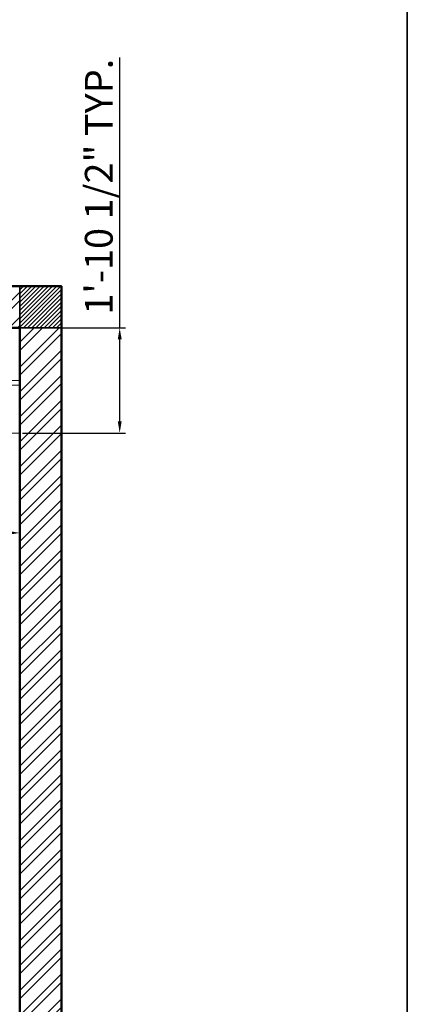
# Model space of a CAD drawing. Units: millimetres. Extents: x 20768 to 23556, y 50760 to 52704.
# Tile 29 of 36: x 21551 to 21634, y 52368 to 52580. Entities that reach past the tile are written whole.
import ezdxf

# ---------------------------------------------------------------- set-up
doc = ezdxf.new("R2010")
doc.units = ezdxf.units.MM
for name, color, linetype, lineweight in [('A-ANNO-TTLB', 7, 'Continuous', 35), ('A-FURN', 8, 'Continuous', 18), ('A-WALL', 7, 'Continuous', 50), ('A-WALL-PATT', 8, 'Continuous', 13), ('S-ANNO-DIMS', 2, 'Continuous', 18), ('S-COLS', 20, 'Continuous', 35)]:
    doc.layers.add(name, color=color, linetype=linetype, lineweight=lineweight)
doc.styles.get("Standard").update_dxf_attribs({"font": 'arial.ttf'})
doc.dimstyles.new('ISO-25', dxfattribs={"dimtxt": 6, "dimasz": 2.5, "dimexe": 1.25, "dimexo": 0.625, "dimtad": 1, "dimdec": 0, "dimlunit": 3, "dimtxsty": 'Standard', "dimcen": 2.5, "dimadec": 0, "dimazin": 0, "dimtfac": 1, "dimtdec": 0, "dimtmove": 0, "dimatfit": 3, "dimfxl": 1, "dimarcsym": 0})
pattern_1 = [(45, (-37.4434, 0), (-2.69407684, 2.69407684), []), (45, (-35.6473, 0), (-2.69407684, 2.69407684), [])]

# ---------------------------------------------------------------- blocks, each defined once
blk = doc.blocks.new('wb')
for p, q in [((21205.25, 52502.52), (21061.44, 52502.52)), ((21205.25, 52501.52), (21061.44, 52501.52))]:
    blk.add_line(p, q)
blk.add_lwpolyline([(21205.25, 52513.9), (21061.44, 52513.9), (21061.44, 52491.15), (21205.25, 52491.15)], close=True)
for points in [[(21064.45, 52510.07, 0.695903), (21063.5, 52509.77), (21063.75, 52508.98), (21064.7, 52509.27)], [(21067.97, 52510.07, 0.695903), (21067.01, 52509.77), (21067.26, 52508.98), (21068.21, 52509.27)], [(21071.48, 52510.07, 0.695903), (21070.52, 52509.77), (21070.77, 52508.98), (21071.73, 52509.27)], [(21074.99, 52510.07, 0.695903), (21074.04, 52509.77), (21074.28, 52508.98), (21075.24, 52509.27)], [(21078.5, 52510.07, 0.695903), (21077.55, 52509.77), (21077.8, 52508.98), (21078.75, 52509.27)], [(21082.02, 52510.07, 0.695903), (21081.06, 52509.77), (21081.31, 52508.98), (21082.26, 52509.27)], [(21085.53, 52510.07, 0.695903), (21084.57, 52509.77), (21084.82, 52508.98), (21085.78, 52509.27)], [(21089.04, 52510.07, 0.695903), (21088.09, 52509.77), (21088.33, 52508.98), (21089.29, 52509.27)], [(21092.55, 52510.07, 0.695903), (21091.6, 52509.77), (21091.85, 52508.98), (21092.8, 52509.27)], [(21096.07, 52510.07, 0.695903), (21095.11, 52509.77), (21095.36, 52508.98), (21096.31, 52509.27)], [(21099.58, 52510.07, 0.695903), (21098.62, 52509.77), (21098.87, 52508.98), (21099.83, 52509.27)], [(21103.09, 52510.07, 0.695903), (21102.14, 52509.77), (21102.38, 52508.98), (21103.34, 52509.27)], [(21106.6, 52510.07, 0.695903), (21105.65, 52509.77), (21105.9, 52508.98), (21106.85, 52509.27)], [(21110.12, 52510.07, 0.695903), (21109.16, 52509.77), (21109.41, 52508.98), (21110.36, 52509.27)], [(21113.63, 52510.07, 0.695903), (21112.67, 52509.77), (21112.92, 52508.98), (21113.88, 52509.27)], [(21117.14, 52510.07, 0.695903), (21116.19, 52509.77), (21116.43, 52508.98), (21117.39, 52509.27)], [(21120.65, 52510.07, 0.695903), (21119.7, 52509.77), (21119.95, 52508.98), (21120.9, 52509.27)], [(21124.17, 52510.07, 0.695903), (21123.21, 52509.77), (21123.46, 52508.98), (21124.41, 52509.27)], [(21127.68, 52510.07, 0.695903), (21126.72, 52509.77), (21126.97, 52508.98), (21127.93, 52509.27)], [(21131.19, 52510.07, 0.695903), (21130.24, 52509.77), (21130.48, 52508.98), (21131.44, 52509.27)], [(21134.7, 52510.07, 0.695903), (21133.75, 52509.77), (21134, 52508.98), (21134.95, 52509.27)], [(21138.22, 52510.07, 0.695903), (21137.26, 52509.77), (21137.51, 52508.98), (21138.46, 52509.27)], [(21141.73, 52510.07, 0.695903), (21140.77, 52509.77), (21141.02, 52508.98), (21141.98, 52509.27)], [(21145.24, 52510.07, 0.695903), (21144.29, 52509.77), (21144.54, 52508.98), (21145.49, 52509.27)], [(21148.75, 52510.07, 0.695903), (21147.8, 52509.77), (21148.05, 52508.98), (21149, 52509.27)], [(21152.27, 52510.07, 0.695903), (21151.31, 52509.77), (21151.56, 52508.98), (21152.52, 52509.27)], [(21155.78, 52510.07, 0.695903), (21154.83, 52509.77), (21155.07, 52508.98), (21156.03, 52509.27)], [(21159.29, 52510.07, 0.695903), (21158.34, 52509.77), (21158.59, 52508.98), (21159.54, 52509.27)], [(21162.8, 52510.07, 0.695903), (21161.85, 52509.77), (21162.1, 52508.98), (21163.05, 52509.27)], [(21166.32, 52510.07, 0.695903), (21165.36, 52509.77), (21165.61, 52508.98), (21166.57, 52509.27)], [(21169.83, 52510.07, 0.695903), (21168.88, 52509.77), (21169.12, 52508.98), (21170.08, 52509.27)], [(21173.34, 52510.07, 0.695903), (21172.39, 52509.77), (21172.64, 52508.98), (21173.59, 52509.27)], [(21176.86, 52510.07, 0.695903), (21175.9, 52509.77), (21176.15, 52508.98), (21177.1, 52509.27)], [(21180.37, 52510.07, 0.695903), (21179.41, 52509.77), (21179.66, 52508.98), (21180.62, 52509.27)], [(21183.88, 52510.07, 0.695903), (21182.93, 52509.77), (21183.17, 52508.98), (21184.13, 52509.27)], [(21187.39, 52510.07, 0.695903), (21186.44, 52509.77), (21186.69, 52508.98), (21187.64, 52509.27)], [(21190.91, 52510.07, 0.695903), (21189.95, 52509.77), (21190.2, 52508.98), (21191.15, 52509.27)], [(21194.42, 52510.07, 0.695903), (21193.46, 52509.77), (21193.71, 52508.98), (21194.67, 52509.27)], [(21197.93, 52510.07, 0.695903), (21196.98, 52509.77), (21197.22, 52508.98), (21198.18, 52509.27)], [(21068.81, 52496.1), (21067.85, 52495.8), (21068.19, 52494.73, 1), (21069.14, 52495.03)], [(21072.32, 52496.1), (21071.37, 52495.8), (21071.7, 52494.73, 1), (21072.65, 52495.03)], [(21075.83, 52496.1), (21074.88, 52495.8), (21075.21, 52494.73, 1), (21076.17, 52495.03)], [(21079.35, 52496.1), (21078.39, 52495.8), (21078.73, 52494.73, 1), (21079.68, 52495.03)], [(21082.86, 52496.1), (21081.9, 52495.8), (21082.24, 52494.73, 1), (21083.19, 52495.03)], [(21086.37, 52496.1), (21085.42, 52495.8), (21085.75, 52494.73, 1), (21086.7, 52495.03)], [(21089.88, 52496.1), (21088.93, 52495.8), (21089.26, 52494.73, 1), (21090.22, 52495.03)], [(21093.4, 52496.1), (21092.44, 52495.8), (21092.78, 52494.73, 1), (21093.73, 52495.03)], [(21096.91, 52496.1), (21095.95, 52495.8), (21096.29, 52494.73, 1), (21097.24, 52495.03)], [(21100.42, 52496.1), (21099.47, 52495.8), (21099.8, 52494.73, 1), (21100.76, 52495.03)], [(21103.93, 52496.1), (21102.98, 52495.8), (21103.31, 52494.73, 1), (21104.27, 52495.03)], [(21107.45, 52496.1), (21106.49, 52495.8), (21106.83, 52494.73, 1), (21107.78, 52495.03)], [(21110.96, 52496.1), (21110, 52495.8), (21110.34, 52494.73, 1), (21111.29, 52495.03)], [(21114.47, 52496.1), (21113.52, 52495.8), (21113.85, 52494.73, 1), (21114.81, 52495.03)], [(21117.98, 52496.1), (21117.03, 52495.8), (21117.36, 52494.73, 1), (21118.32, 52495.03)], [(21121.5, 52496.1), (21120.54, 52495.8), (21120.88, 52494.73, 1), (21121.83, 52495.03)], [(21125.01, 52496.1), (21124.05, 52495.8), (21124.39, 52494.73, 1), (21125.34, 52495.03)], [(21128.52, 52496.1), (21127.57, 52495.8), (21127.9, 52494.73, 1), (21128.86, 52495.03)], [(21132.03, 52496.1), (21131.08, 52495.8), (21131.41, 52494.73, 1), (21132.37, 52495.03)], [(21135.55, 52496.1), (21134.59, 52495.8), (21134.93, 52494.73, 1), (21135.88, 52495.03)], [(21139.06, 52496.1), (21138.1, 52495.8), (21138.44, 52494.73, 1), (21139.39, 52495.03)], [(21142.57, 52496.1), (21141.62, 52495.8), (21141.95, 52494.73, 1), (21142.91, 52495.03)], [(21146.08, 52496.1), (21145.13, 52495.8), (21145.46, 52494.73, 1), (21146.42, 52495.03)], [(21149.6, 52496.1), (21148.64, 52495.8), (21148.98, 52494.73, 1), (21149.93, 52495.03)], [(21153.11, 52496.1), (21152.15, 52495.8), (21152.49, 52494.73, 1), (21153.44, 52495.03)], [(21156.62, 52496.1), (21155.67, 52495.8), (21156, 52494.73, 1), (21156.96, 52495.03)], [(21160.13, 52496.1), (21159.18, 52495.8), (21159.51, 52494.73, 1), (21160.47, 52495.03)], [(21163.65, 52496.1), (21162.69, 52495.8), (21163.03, 52494.73, 1), (21163.98, 52495.03)], [(21167.16, 52496.1), (21166.2, 52495.8), (21166.54, 52494.73, 1), (21167.49, 52495.03)], [(21170.67, 52496.1), (21169.72, 52495.8), (21170.05, 52494.73, 1), (21171.01, 52495.03)], [(21174.18, 52496.1), (21173.23, 52495.8), (21173.56, 52494.73, 1), (21174.52, 52495.03)], [(21177.7, 52496.1), (21176.74, 52495.8), (21177.08, 52494.73, 1), (21178.03, 52495.03)], [(21181.21, 52496.1), (21180.25, 52495.8), (21180.59, 52494.73, 1), (21181.54, 52495.03)], [(21184.72, 52496.1), (21183.77, 52495.8), (21184.1, 52494.73, 1), (21185.06, 52495.03)], [(21188.23, 52496.1), (21187.28, 52495.8), (21187.61, 52494.73, 1), (21188.57, 52495.03)], [(21191.75, 52496.1), (21190.79, 52495.8), (21191.13, 52494.73, 1), (21192.08, 52495.03)], [(21195.26, 52496.1), (21194.31, 52495.8), (21194.64, 52494.73, 1), (21195.59, 52495.03)], [(21198.77, 52496.1), (21197.82, 52495.8), (21198.15, 52494.73, 1), (21199.11, 52495.03)], [(21202.29, 52496.1), (21201.33, 52495.8), (21201.67, 52494.73, 1), (21202.62, 52495.03)]]:
    blk.add_lwpolyline(points, format="xyb", close=True)
for points in [[(21065.76, 52502.52), (21063.98, 52508.23), (21064.93, 52508.53), (21066.81, 52502.52)], [(21069.27, 52502.52), (21067.49, 52508.23), (21068.44, 52508.53), (21070.32, 52502.52)], [(21072.78, 52502.52), (21071, 52508.23), (21071.96, 52508.53), (21073.83, 52502.52)], [(21076.3, 52502.52), (21074.51, 52508.23), (21075.47, 52508.53), (21077.34, 52502.52)], [(21079.81, 52502.52), (21078.03, 52508.23), (21078.98, 52508.53), (21080.86, 52502.52)], [(21083.32, 52502.52), (21081.54, 52508.23), (21082.49, 52508.53), (21084.37, 52502.52)], [(21086.83, 52502.52), (21085.05, 52508.23), (21086.01, 52508.53), (21087.88, 52502.52)], [(21090.35, 52502.52), (21088.57, 52508.23), (21089.52, 52508.53), (21091.39, 52502.52)], [(21093.86, 52502.52), (21092.08, 52508.23), (21093.03, 52508.53), (21094.91, 52502.52)], [(21097.37, 52502.52), (21095.59, 52508.23), (21096.55, 52508.53), (21098.42, 52502.52)], [(21100.88, 52502.52), (21099.1, 52508.23), (21100.06, 52508.53), (21101.93, 52502.52)], [(21104.4, 52502.52), (21102.62, 52508.23), (21103.57, 52508.53), (21105.44, 52502.52)], [(21107.91, 52502.52), (21106.13, 52508.23), (21107.08, 52508.53), (21108.96, 52502.52)], [(21111.42, 52502.52), (21109.64, 52508.23), (21110.6, 52508.53), (21112.47, 52502.52)], [(21114.93, 52502.52), (21113.15, 52508.23), (21114.11, 52508.53), (21115.98, 52502.52)], [(21118.45, 52502.52), (21116.67, 52508.23), (21117.62, 52508.53), (21119.49, 52502.52)], [(21121.96, 52502.52), (21120.18, 52508.23), (21121.13, 52508.53), (21123.01, 52502.52)], [(21125.47, 52502.52), (21123.69, 52508.23), (21124.65, 52508.53), (21126.52, 52502.52)], [(21128.98, 52502.52), (21127.2, 52508.23), (21128.16, 52508.53), (21130.03, 52502.52)], [(21132.5, 52502.52), (21130.72, 52508.23), (21131.67, 52508.53), (21133.54, 52502.52)], [(21136.01, 52502.52), (21134.23, 52508.23), (21135.18, 52508.53), (21137.06, 52502.52)], [(21139.52, 52502.52), (21137.74, 52508.23), (21138.7, 52508.53), (21140.57, 52502.52)], [(21143.03, 52502.52), (21141.25, 52508.23), (21142.21, 52508.53), (21144.08, 52502.52)], [(21146.55, 52502.52), (21144.77, 52508.23), (21145.72, 52508.53), (21147.59, 52502.52)], [(21150.06, 52502.52), (21148.28, 52508.23), (21149.23, 52508.53), (21151.11, 52502.52)], [(21153.57, 52502.52), (21151.79, 52508.23), (21152.75, 52508.53), (21154.62, 52502.52)], [(21157.08, 52502.52), (21155.3, 52508.23), (21156.26, 52508.53), (21158.13, 52502.52)], [(21160.6, 52502.52), (21158.82, 52508.23), (21159.77, 52508.53), (21161.64, 52502.52)], [(21164.11, 52502.52), (21162.33, 52508.23), (21163.28, 52508.53), (21165.16, 52502.52)], [(21167.62, 52502.52), (21165.84, 52508.23), (21166.8, 52508.53), (21168.67, 52502.52)], [(21171.13, 52502.52), (21169.35, 52508.23), (21170.31, 52508.53), (21172.18, 52502.52)], [(21174.65, 52502.52), (21172.87, 52508.23), (21173.82, 52508.53), (21175.69, 52502.52)], [(21178.16, 52502.52), (21176.38, 52508.23), (21177.33, 52508.53), (21179.21, 52502.52)], [(21181.67, 52502.52), (21179.89, 52508.23), (21180.85, 52508.53), (21182.72, 52502.52)], [(21185.19, 52502.52), (21183.4, 52508.23), (21184.36, 52508.53), (21186.23, 52502.52)], [(21188.7, 52502.52), (21186.92, 52508.23), (21187.87, 52508.53), (21189.75, 52502.52)], [(21192.21, 52502.52), (21190.43, 52508.23), (21191.38, 52508.53), (21193.26, 52502.52)], [(21195.72, 52502.52), (21193.94, 52508.23), (21194.9, 52508.53), (21196.77, 52502.52)], [(21199.24, 52502.52), (21197.46, 52508.23), (21198.41, 52508.53), (21200.28, 52502.52)], [(21066.07, 52501.52), (21067.54, 52496.81), (21068.49, 52497.1), (21067.12, 52501.52)], [(21069.58, 52501.52), (21071.05, 52496.81), (21072.01, 52497.1), (21070.63, 52501.52)], [(21073.09, 52501.52), (21074.57, 52496.81), (21075.52, 52497.1), (21074.14, 52501.52)], [(21076.61, 52501.52), (21078.08, 52496.81), (21079.03, 52497.1), (21077.65, 52501.52)], [(21080.12, 52501.52), (21081.59, 52496.81), (21082.55, 52497.1), (21081.17, 52501.52)], [(21083.63, 52501.52), (21085.1, 52496.81), (21086.06, 52497.1), (21084.68, 52501.52)], [(21087.14, 52501.52), (21088.62, 52496.81), (21089.57, 52497.1), (21088.19, 52501.52)], [(21090.66, 52501.52), (21092.13, 52496.81), (21093.08, 52497.1), (21091.7, 52501.52)], [(21094.17, 52501.52), (21095.64, 52496.81), (21096.6, 52497.1), (21095.22, 52501.52)], [(21097.68, 52501.52), (21099.15, 52496.81), (21100.11, 52497.1), (21098.73, 52501.52)], [(21101.2, 52501.52), (21102.67, 52496.81), (21103.62, 52497.1), (21102.24, 52501.52)], [(21104.71, 52501.52), (21106.18, 52496.81), (21107.13, 52497.1), (21105.76, 52501.52)], [(21108.22, 52501.52), (21109.69, 52496.81), (21110.65, 52497.1), (21109.27, 52501.52)], [(21111.73, 52501.52), (21113.2, 52496.81), (21114.16, 52497.1), (21112.78, 52501.52)], [(21115.25, 52501.52), (21116.72, 52496.81), (21117.67, 52497.1), (21116.29, 52501.52)], [(21118.76, 52501.52), (21120.23, 52496.81), (21121.18, 52497.1), (21119.81, 52501.52)], [(21122.27, 52501.52), (21123.74, 52496.81), (21124.7, 52497.1), (21123.32, 52501.52)], [(21125.78, 52501.52), (21127.25, 52496.81), (21128.21, 52497.1), (21126.83, 52501.52)], [(21129.3, 52501.52), (21130.77, 52496.81), (21131.72, 52497.1), (21130.34, 52501.52)], [(21132.81, 52501.52), (21134.28, 52496.81), (21135.23, 52497.1), (21133.86, 52501.52)], [(21136.32, 52501.52), (21137.79, 52496.81), (21138.75, 52497.1), (21137.37, 52501.52)], [(21139.83, 52501.52), (21141.3, 52496.81), (21142.26, 52497.1), (21140.88, 52501.52)], [(21143.35, 52501.52), (21144.82, 52496.81), (21145.77, 52497.1), (21144.39, 52501.52)], [(21146.86, 52501.52), (21148.33, 52496.81), (21149.28, 52497.1), (21147.91, 52501.52)], [(21150.37, 52501.52), (21151.84, 52496.81), (21152.8, 52497.1), (21151.42, 52501.52)], [(21153.88, 52501.52), (21155.35, 52496.81), (21156.31, 52497.1), (21154.93, 52501.52)], [(21157.4, 52501.52), (21158.87, 52496.81), (21159.82, 52497.1), (21158.44, 52501.52)], [(21160.91, 52501.52), (21162.38, 52496.81), (21163.33, 52497.1), (21161.96, 52501.52)], [(21164.42, 52501.52), (21165.89, 52496.81), (21166.85, 52497.1), (21165.47, 52501.52)], [(21167.93, 52501.52), (21169.4, 52496.81), (21170.36, 52497.1), (21168.98, 52501.52)], [(21171.45, 52501.52), (21172.92, 52496.81), (21173.87, 52497.1), (21172.49, 52501.52)], [(21174.96, 52501.52), (21176.43, 52496.81), (21177.38, 52497.1), (21176.01, 52501.52)], [(21178.47, 52501.52), (21179.94, 52496.81), (21180.9, 52497.1), (21179.52, 52501.52)], [(21181.98, 52501.52), (21183.46, 52496.81), (21184.41, 52497.1), (21183.03, 52501.52)], [(21185.5, 52501.52), (21186.97, 52496.81), (21187.92, 52497.1), (21186.54, 52501.52)], [(21189.01, 52501.52), (21190.48, 52496.81), (21191.43, 52497.1), (21190.06, 52501.52)], [(21192.52, 52501.52), (21193.99, 52496.81), (21194.95, 52497.1), (21193.57, 52501.52)], [(21196.03, 52501.52), (21197.51, 52496.81), (21198.46, 52497.1), (21197.08, 52501.52)], [(21199.55, 52501.52), (21201.02, 52496.81), (21201.97, 52497.1), (21200.59, 52501.52)]]:
    blk.add_lwpolyline(points)
blk = doc.blocks.new('*D187')
at = {"layer": 'Defpoints', "color": 0, "transparency": 16777216}
for p in [(21406.93, 52491.15), (21550.74, 52491.15), (21550.74, 52469.58)]:
    blk.add_point(p, dxfattribs=at)
at = {"layer": 'S-ANNO-DIMS', "color": 0, "lineweight": -2, "transparency": 16777216}
for p, q in [((21406.93, 52490.53), (21406.93, 52468.33)), ((21550.74, 52490.53), (21550.74, 52468.33)), ((21409.43, 52469.58), (21548.24, 52469.58))]:
    blk.add_line(p, q, dxfattribs=at)
at = {"layer": 'S-ANNO-DIMS', "color": 0, "transparency": 16777216}
for points in [[(21409.43, 52470), (21409.43, 52469.16), (21406.93, 52469.58)], [(21548.24, 52470), (21548.24, 52469.16), (21550.74, 52469.58)]]:
    blk.add_solid(points, dxfattribs=at)
at = {"layer": 'S-ANNO-DIMS', "color": 0, "transparency": 16777216, "insert": (21478.84, 52473.31), "char_height": 6, "attachment_point": 5}
blk.add_mtext('WARDROBE 12\'-0" TYP.', dxfattribs=at)
blk = doc.blocks.new('*D188')
at = {"layer": 'Defpoints', "color": 0, "transparency": 16777216}
for p in [(21550.74, 52513.9), (21572.31, 52513.9), (21550.74, 52491.15)]:
    blk.add_point(p, dxfattribs=at)
at = {"layer": 'S-ANNO-DIMS', "color": 0, "lineweight": -2, "transparency": 16777216}
for p, q in [((21572.31, 52513.9), (21572.31, 52572.3)), ((21551.37, 52513.9), (21573.56, 52513.9)), ((21572.31, 52493.65), (21572.31, 52511.4)), ((21551.37, 52491.15), (21573.56, 52491.15))]:
    blk.add_line(p, q, dxfattribs=at)
at = {"layer": 'S-ANNO-DIMS', "color": 0, "transparency": 16777216}
for points in [[(21571.9, 52511.4), (21572.73, 52511.4), (21572.31, 52513.9)], [(21571.9, 52493.65), (21572.73, 52493.65), (21572.31, 52491.15)]]:
    blk.add_solid(points, dxfattribs=at)
at = {"layer": 'S-ANNO-DIMS', "color": 0, "transparency": 16777216, "insert": (21568.58, 52544.35), "char_height": 6, "attachment_point": 5, "rotation": 90}
blk.add_mtext('1\'-10 1/2" TYP.', dxfattribs=at)

msp = doc.modelspace()

# ---------------------------------------------------------------- hatches: boundary and pattern name
at = {"layer": 'A-WALL-PATT'}
h = msp.add_hatch(dxfattribs=at)
h.set_pattern_fill('ANSI32', color=256, scale=0.4)
h.set_pattern_definition(pattern_1)
h.paths.add_polyline_path([(21550.74, 52522.9), (21334.74, 52522.9), (21334.74, 52513.9), (21550.74, 52513.9)])
h = msp.add_hatch(dxfattribs=at)
h.set_pattern_fill('ANSI31', color=256, scale=0.2)
h.set_pattern_definition([(45, (345.4904, 0), (-0.449012806, 0.449012806), [])])
h.paths.add_polyline_path([(21559.74, 52522.9), (21550.74, 52522.9), (21550.74, 52513.9), (21559.74, 52513.9)])
h = msp.add_hatch(dxfattribs=at)
h.set_pattern_fill('ANSI32', color=256, scale=0.4)
h.set_pattern_definition(pattern_1)
h.paths.add_polyline_path([(21559.74, 52513.9), (21550.74, 52513.9), (21550.74, 52335.9), (21559.74, 52335.9)])

# ---------------------------------------------------------------- linework, layer by layer
at = {"layer": 'A-ANNO-TTLB'}
msp.add_line((21634.36, 52703.98), (21634.36, 51623.53), dxfattribs=at)
at = {"layer": 'A-WALL'}
for p, q in [((21325.74, 52522.9), (21559.74, 52522.9)), ((21559.74, 52522.9), (21559.74, 51829.9)), ((21334.74, 52513.9), (21550.74, 52513.9)), ((21550.74, 52513.9), (21550.74, 51834.4))]:
    msp.add_line(p, q, dxfattribs=at)
at = {"layer": 'S-COLS'}
msp.add_lwpolyline([(21550.74, 52513.9), (21559.74, 52513.9), (21559.74, 52522.9), (21550.74, 52522.9)], close=True, dxfattribs=at)

# ---------------------------------------------------------------- block references
at = {"layer": 'A-FURN'}
msp.add_blockref('wb', (345.49, 0), dxfattribs=at)

# ---------------------------------------------------------------- dimensions: what is measured, and where the dimension line sits
at = {"layer": 'S-ANNO-DIMS'}
dim = msp.add_linear_dim(base=(21572.3121, 52513.8969), p1=(21550.7411, 52491.1517), p2=(21550.7411, 52513.8969), angle=90, text='<> TYP.', dimstyle='ISO-25', override={"dimdec": 1, "dimrnd": 0, "dimzin": 1, "dimlunit": 4, "dimfrac": 2}, dxfattribs=at)
dim.commit()
dim.dimension.update_dxf_attribs({"geometry": '*D188', "text_midpoint": (21568.5848, 52544.3472)})
dim = msp.add_linear_dim(base=(21550.74, 52469.58), p1=(21406.93, 52491.15), p2=(21550.74, 52491.15), text='WARDROBE <> TYP.', dimstyle='ISO-25', override={"dimdec": 1, "dimrnd": 0, "dimzin": 1, "dimlunit": 4, "dimfrac": 2}, dxfattribs=at)
dim.commit()
dim.dimension.update_dxf_attribs({"geometry": '*D187', "text_midpoint": (21478.84, 52473.31)})

doc.saveas('drawing.dxf')
